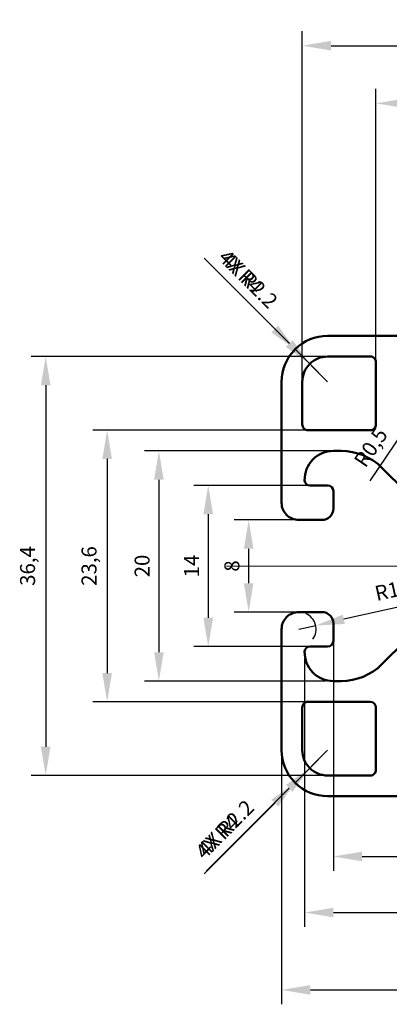
# Model space of a CAD drawing. Units: millimetres. Extents: x 2580.1 to 2672.5, y 2225.2 to 2310.7.
# Tile 1 of 2: x 2580.1 to 2612.2, y 2225.2 to 2310.7. Entities that reach past the tile are written whole.
import ezdxf

# ---------------------------------------------------------------- set-up
doc = ezdxf.new("R2010")
doc.units = ezdxf.units.MM
doc.linetypes.add('CENTER', pattern=[50.8, 31.75, -6.35, 6.35, -6.35])
for name, color, linetype, lineweight in [('M-CNTR', 1, 'CENTER', 18), ('M-DIMS', 2, 'Continuous', 25), ('M-OUTL', 7, 'Continuous', 50)]:
    doc.layers.add(name, color=color, linetype=linetype, lineweight=lineweight)
doc.styles.get("Standard").update_dxf_attribs({"font": 'arial.ttf'})
doc.dimstyles.new('ISO-25', dxfattribs={"dimtxt": 1.3, "dimasz": 2.5, "dimexe": 1.25, "dimexo": 0.625, "dimtad": 1, "dimtxsty": 'Standard', "dimcen": 2.5, "dimadec": 0, "dimazin": 0, "dimtfac": 1, "dimtmove": 0, "dimatfit": 3, "dimfxl": 1, "dimarcsym": 0})

# ---------------------------------------------------------------- blocks, each defined once
blk = doc.blocks.new('*D4')
at = {"layer": 'Defpoints', "color": 0, "transparency": 16777216}
for p in [(2634.649, 2303.442), (2611.049, 2278.243), (2634.649, 2278.243)]:
    blk.add_point(p, dxfattribs=at)
at = {"layer": 'M-DIMS', "color": 0, "lineweight": -2, "transparency": 16777216}
for p, q in [((2611.049, 2278.868), (2611.049, 2304.692)), ((2634.649, 2278.868), (2634.649, 2304.692)), ((2613.549, 2303.442), (2632.149, 2303.442))]:
    blk.add_line(p, q, dxfattribs=at)
at = {"layer": 'M-DIMS', "color": 0, "transparency": 16777216}
for points in [[(2613.549, 2303.859), (2613.549, 2303.026), (2611.049, 2303.442)], [(2632.149, 2303.859), (2632.149, 2303.026), (2634.649, 2303.442)]]:
    blk.add_solid(points, dxfattribs=at)
at = {"layer": 'M-DIMS', "color": 0, "transparency": 16777216, "insert": (2622.849, 2304.849), "char_height": 1.3, "attachment_point": 5}
blk.add_mtext('23,6', dxfattribs=at)
blk = doc.blocks.new('*D5')
at = {"layer": 'Defpoints', "color": 0, "transparency": 16777216}
for p in [(2641.049, 2308.452), (2604.649, 2277.393), (2641.049, 2277.393)]:
    blk.add_point(p, dxfattribs=at)
at = {"layer": 'M-DIMS', "color": 0, "lineweight": -2, "transparency": 16777216}
for p, q in [((2604.649, 2278.018), (2604.649, 2309.702)), ((2641.049, 2278.018), (2641.049, 2309.702)), ((2607.149, 2308.452), (2638.549, 2308.452))]:
    blk.add_line(p, q, dxfattribs=at)
at = {"layer": 'M-DIMS', "color": 0, "transparency": 16777216}
for points in [[(2607.149, 2308.869), (2607.149, 2308.036), (2604.649, 2308.452)], [(2638.549, 2308.869), (2638.549, 2308.036), (2641.049, 2308.452)]]:
    blk.add_solid(points, dxfattribs=at)
at = {"layer": 'M-DIMS', "color": 0, "transparency": 16777216, "insert": (2622.849, 2309.859), "char_height": 1.3, "attachment_point": 5}
blk.add_mtext('36,4', dxfattribs=at)
blk = doc.blocks.new('*D6')
at = {"layer": 'Defpoints', "color": 0, "transparency": 16777216}
for p in [(2608.699, 2281.443), (2582.357, 2245.043), (2608.699, 2245.043)]:
    blk.add_point(p, dxfattribs=at)
at = {"layer": 'M-DIMS', "color": 0, "lineweight": -2, "transparency": 16777216}
for p, q in [((2608.074, 2281.443), (2581.107, 2281.443)), ((2582.357, 2278.943), (2582.357, 2247.543)), ((2608.074, 2245.043), (2581.107, 2245.043))]:
    blk.add_line(p, q, dxfattribs=at)
at = {"layer": 'M-DIMS', "color": 0, "transparency": 16777216}
for points in [[(2581.941, 2278.943), (2582.774, 2278.943), (2582.357, 2281.443)], [(2581.941, 2247.543), (2582.774, 2247.543), (2582.357, 2245.043)]]:
    blk.add_solid(points, dxfattribs=at)
at = {"layer": 'M-DIMS', "color": 0, "transparency": 16777216, "insert": (2580.951, 2263.243), "char_height": 1.3, "attachment_point": 5, "rotation": 90}
blk.add_mtext('36,4', dxfattribs=at)
blk = doc.blocks.new('*D7')
at = {"layer": 'Defpoints', "color": 0, "transparency": 16777216}
for p in [(2605.349, 2267.243), (2599.989, 2259.243), (2605.349, 2259.243)]:
    blk.add_point(p, dxfattribs=at)
at = {"layer": 'M-DIMS', "color": 0, "lineweight": -2, "transparency": 16777216}
for p, q in [((2604.724, 2267.243), (2598.739, 2267.243)), ((2599.989, 2264.743), (2599.989, 2261.743)), ((2604.724, 2259.243), (2598.739, 2259.243))]:
    blk.add_line(p, q, dxfattribs=at)
at = {"layer": 'M-DIMS', "color": 0, "transparency": 16777216}
for points in [[(2599.572, 2264.743), (2600.405, 2264.743), (2599.989, 2267.243)], [(2599.572, 2261.743), (2600.405, 2261.743), (2599.989, 2259.243)]]:
    blk.add_solid(points, dxfattribs=at)
at = {"layer": 'M-DIMS', "color": 0, "transparency": 16777216, "insert": (2598.7, 2263.243), "char_height": 1.3, "attachment_point": 5, "rotation": 90}
blk.add_mtext('8', dxfattribs=at)
blk = doc.blocks.new('*D8')
at = {"layer": 'Defpoints', "color": 0, "transparency": 16777216}
for p in [(2606.075, 2270.243), (2596.476, 2256.243), (2606.075, 2256.243)]:
    blk.add_point(p, dxfattribs=at)
at = {"layer": 'M-DIMS', "color": 0, "lineweight": -2, "transparency": 16777216}
for p, q in [((2605.45, 2270.243), (2595.226, 2270.243)), ((2596.476, 2267.743), (2596.476, 2258.743)), ((2605.45, 2256.243), (2595.226, 2256.243))]:
    blk.add_line(p, q, dxfattribs=at)
at = {"layer": 'M-DIMS', "color": 0, "transparency": 16777216}
for points in [[(2596.06, 2267.743), (2596.893, 2267.743), (2596.476, 2270.243)], [(2596.06, 2258.743), (2596.893, 2258.743), (2596.476, 2256.243)]]:
    blk.add_solid(points, dxfattribs=at)
at = {"layer": 'M-DIMS', "color": 0, "transparency": 16777216, "insert": (2595.199, 2263.243), "char_height": 1.3, "attachment_point": 5, "rotation": 90}
blk.add_mtext('14', dxfattribs=at)
blk = doc.blocks.new('*D9')
at = {"layer": 'Defpoints', "color": 0, "transparency": 16777216}
for p in [(2607.689, 2273.243), (2592.189, 2253.244), (2607.301, 2253.244)]:
    blk.add_point(p, dxfattribs=at)
at = {"layer": 'M-DIMS', "color": 0, "lineweight": -2, "transparency": 16777216}
for p, q in [((2607.064, 2273.243), (2590.939, 2273.243)), ((2592.189, 2270.743), (2592.189, 2255.744)), ((2606.676, 2253.244), (2590.939, 2253.244))]:
    blk.add_line(p, q, dxfattribs=at)
at = {"layer": 'M-DIMS', "color": 0, "transparency": 16777216}
for points in [[(2591.773, 2270.743), (2592.606, 2270.743), (2592.189, 2273.243)], [(2591.773, 2255.744), (2592.606, 2255.744), (2592.189, 2253.244)]]:
    blk.add_solid(points, dxfattribs=at)
at = {"layer": 'M-DIMS', "color": 0, "transparency": 16777216, "insert": (2590.901, 2263.244), "char_height": 1.3, "attachment_point": 5, "rotation": 90}
blk.add_mtext('20', dxfattribs=at)
blk = doc.blocks.new('*D10')
at = {"layer": 'Defpoints', "color": 0, "transparency": 16777216}
for p in [(2607.849, 2275.043), (2587.696, 2251.443), (2607.849, 2251.443)]:
    blk.add_point(p, dxfattribs=at)
at = {"layer": 'M-DIMS', "color": 0, "lineweight": -2, "transparency": 16777216}
for p, q in [((2607.224, 2275.043), (2586.446, 2275.043)), ((2587.696, 2272.543), (2587.696, 2253.943)), ((2607.224, 2251.443), (2586.446, 2251.443))]:
    blk.add_line(p, q, dxfattribs=at)
at = {"layer": 'M-DIMS', "color": 0, "transparency": 16777216}
for points in [[(2587.279, 2272.543), (2588.113, 2272.543), (2587.696, 2275.043)], [(2587.279, 2253.943), (2588.113, 2253.943), (2587.696, 2251.443)]]:
    blk.add_solid(points, dxfattribs=at)
at = {"layer": 'M-DIMS', "color": 0, "transparency": 16777216, "insert": (2586.29, 2263.243), "char_height": 1.3, "attachment_point": 5, "rotation": 90}
blk.add_mtext('23,6', dxfattribs=at)
blk = doc.blocks.new('*D11')
at = {"layer": 'Defpoints', "color": 0, "transparency": 16777216}
for p in [(2602.849, 2247.243), (2642.849, 2247.243), (2642.849, 2226.409)]:
    blk.add_point(p, dxfattribs=at)
at = {"layer": 'M-DIMS', "color": 0, "lineweight": -2, "transparency": 16777216}
for p, q in [((2602.849, 2246.618), (2602.849, 2225.159)), ((2642.849, 2246.618), (2642.849, 2225.159)), ((2605.349, 2226.409), (2640.349, 2226.409))]:
    blk.add_line(p, q, dxfattribs=at)
at = {"layer": 'M-DIMS', "color": 0, "transparency": 16777216}
for points in [[(2605.349, 2226.826), (2605.349, 2225.992), (2602.849, 2226.409)], [(2640.349, 2226.826), (2640.349, 2225.992), (2642.849, 2226.409)]]:
    blk.add_solid(points, dxfattribs=at)
at = {"layer": 'M-DIMS', "color": 0, "transparency": 16777216, "insert": (2622.849, 2227.698), "char_height": 1.3, "attachment_point": 5}
blk.add_mtext('40', dxfattribs=at)
blk = doc.blocks.new('*D12')
at = {"layer": 'Defpoints', "color": 0, "transparency": 16777216}
for p in [(2607.349, 2257.493), (2638.349, 2257.493), (2638.349, 2238.001)]:
    blk.add_point(p, dxfattribs=at)
at = {"layer": 'M-DIMS', "color": 0, "lineweight": -2, "transparency": 16777216}
for p, q in [((2607.349, 2256.868), (2607.349, 2236.751)), ((2638.349, 2256.868), (2638.349, 2236.751)), ((2609.849, 2238.001), (2635.849, 2238.001))]:
    blk.add_line(p, q, dxfattribs=at)
at = {"layer": 'M-DIMS', "color": 0, "transparency": 16777216}
for points in [[(2609.849, 2238.418), (2609.849, 2237.584), (2607.349, 2238.001)], [(2635.849, 2238.418), (2635.849, 2237.584), (2638.349, 2238.001)]]:
    blk.add_solid(points, dxfattribs=at)
at = {"layer": 'M-DIMS', "color": 0, "transparency": 16777216, "insert": (2622.849, 2239.29), "char_height": 1.3, "attachment_point": 5}
blk.add_mtext('31', dxfattribs=at)
blk = doc.blocks.new('*D13')
at = {"layer": 'Defpoints', "color": 0, "transparency": 16777216}
for p in [(2604.85, 2255.804), (2640.849, 2255.743), (2640.849, 2233.131)]:
    blk.add_point(p, dxfattribs=at)
at = {"layer": 'M-DIMS', "color": 0, "lineweight": -2, "transparency": 16777216}
for p, q in [((2604.85, 2255.179), (2604.85, 2231.881)), ((2640.849, 2255.118), (2640.849, 2231.881)), ((2607.35, 2233.131), (2638.349, 2233.131))]:
    blk.add_line(p, q, dxfattribs=at)
at = {"layer": 'M-DIMS', "color": 0, "transparency": 16777216}
for points in [[(2607.35, 2233.547), (2607.35, 2232.714), (2604.85, 2233.131)], [(2638.349, 2233.547), (2638.349, 2232.714), (2640.849, 2233.131)]]:
    blk.add_solid(points, dxfattribs=at)
at = {"layer": 'M-DIMS', "color": 0, "transparency": 16777216, "insert": (2622.85, 2234.42), "char_height": 1.3, "attachment_point": 5}
blk.add_mtext('36', dxfattribs=at)
blk = doc.blocks.new('*D18')
at = {"layer": 'Defpoints', "color": 0, "transparency": 16777216}
for p in [(2616.349, 2279.243), (2616.069, 2278.829)]:
    blk.add_point(p, dxfattribs=at)
at = {"layer": 'M-DIMS', "color": 0, "lineweight": -2, "transparency": 16777216}
for p, q in [((2616.349, 2279.243), (2616.069, 2278.829)), ((2610.54, 2270.653), (2614.669, 2276.758))]:
    blk.add_line(p, q, dxfattribs=at)
at = {"layer": 'M-DIMS', "color": 0, "transparency": 16777216}
blk.add_solid([(2614.324, 2276.992), (2615.014, 2276.525), (2616.069, 2278.829)], dxfattribs=at)
at = {"layer": 'M-DIMS', "color": 0, "transparency": 16777216, "insert": (2610.739, 2273.458), "char_height": 1.3, "attachment_point": 5, "rotation": 55.93249}
blk.add_mtext('R0,5', dxfattribs=at)
blk = doc.blocks.new('*D24')
at = {"layer": 'Defpoints', "color": 0, "transparency": 16777216}
for p in [(2604.349, 2257.743), (2605.814, 2258.069)]:
    blk.add_point(p, dxfattribs=at)
at = {"layer": 'M-DIMS', "color": 0, "lineweight": -2, "transparency": 16777216}
for p, q in [((2615.449, 2260.209), (2608.254, 2258.611)), ((2604.349, 2257.743), (2605.814, 2258.069))]:
    blk.add_line(p, q, dxfattribs=at)
blk.add_arc((2604.349, 2257.743), 1.5, 324.77892, 66.12676, dxfattribs=at)
at = {"layer": 'M-DIMS', "color": 0, "transparency": 16777216}
blk.add_solid([(2608.164, 2259.018), (2608.345, 2258.204), (2605.814, 2258.069)], dxfattribs=at)
at = {"layer": 'M-DIMS', "color": 0, "transparency": 16777216, "insert": (2612.767, 2261.054), "char_height": 1.3, "attachment_point": 5, "rotation": 12.5254}
blk.add_mtext('R1,5', dxfattribs=at)
blk = doc.blocks.new('*D35')
at = {"layer": 'Defpoints', "color": 0, "transparency": 16777216}
for p in [(2606.849, 2247.243), (2604.023, 2244.413)]:
    blk.add_point(p, dxfattribs=at)
at = {"layer": 'M-DIMS', "color": 0, "lineweight": -2, "transparency": 16777216}
for p, q in [((2606.849, 2247.243), (2604.023, 2244.413)), ((2596.118, 2236.497), (2602.256, 2242.644))]:
    blk.add_line(p, q, dxfattribs=at)
at = {"layer": 'M-DIMS', "color": 0, "transparency": 16777216}
blk.add_solid([(2601.962, 2242.938), (2602.551, 2242.35), (2604.023, 2244.413)], dxfattribs=at)
at = {"layer": 'M-DIMS', "color": 0, "transparency": 16777216, "insert": (2597.402, 2239.587), "char_height": 1.3, "attachment_point": 5, "rotation": 45.04}
blk.add_mtext('4X R4', dxfattribs=at)
blk = doc.blocks.new('*D36')
at = {"layer": 'Defpoints', "color": 0, "transparency": 16777216}
for p in [(2606.849, 2247.243), (2605.291, 2245.691)]:
    blk.add_point(p, dxfattribs=at)
at = {"layer": 'M-DIMS', "color": 0, "lineweight": -2, "transparency": 16777216}
for p, q in [((2606.849, 2247.243), (2605.291, 2245.691)), ((2596.298, 2236.733), (2603.52, 2243.926))]:
    blk.add_line(p, q, dxfattribs=at)
at = {"layer": 'M-DIMS', "color": 0, "transparency": 16777216}
blk.add_solid([(2603.226, 2244.222), (2603.814, 2243.631), (2605.291, 2245.691)], dxfattribs=at)
at = {"layer": 'M-DIMS', "color": 0, "transparency": 16777216, "insert": (2598.121, 2240.353), "char_height": 1.3, "attachment_point": 5, "rotation": 44.88871}
blk.add_mtext('4X R2.2', dxfattribs=at)
blk = doc.blocks.new('*D37')
at = {"layer": 'Defpoints', "color": 0, "transparency": 16777216}
for p in [(2604.021, 2282.072), (2606.849, 2279.243)]:
    blk.add_point(p, dxfattribs=at)
at = {"layer": 'M-DIMS', "color": 0, "lineweight": -2, "transparency": 16777216}
for p, q in [((2596.111, 2289.982), (2602.253, 2283.84)), ((2606.849, 2279.243), (2604.021, 2282.072))]:
    blk.add_line(p, q, dxfattribs=at)
at = {"layer": 'M-DIMS', "color": 0, "transparency": 16777216}
blk.add_solid([(2602.548, 2284.134), (2601.959, 2283.545), (2604.021, 2282.072)], dxfattribs=at)
at = {"layer": 'M-DIMS', "color": 0, "transparency": 16777216, "insert": (2599.2, 2288.697), "char_height": 1.3, "attachment_point": 5, "rotation": 314.99783}
blk.add_mtext('4X R4', dxfattribs=at)
blk = doc.blocks.new('*D38')
at = {"layer": 'Defpoints', "color": 0, "transparency": 16777216}
for p in [(2605.294, 2280.799), (2606.849, 2279.243)]:
    blk.add_point(p, dxfattribs=at)
at = {"layer": 'M-DIMS', "color": 0, "lineweight": -2, "transparency": 16777216}
for p, q in [((2596.319, 2289.775), (2603.526, 2282.567)), ((2606.849, 2279.243), (2605.294, 2280.799))]:
    blk.add_line(p, q, dxfattribs=at)
at = {"layer": 'M-DIMS', "color": 0, "transparency": 16777216}
blk.add_solid([(2603.821, 2282.862), (2603.232, 2282.272), (2605.294, 2280.799)], dxfattribs=at)
at = {"layer": 'M-DIMS', "color": 0, "transparency": 16777216, "insert": (2599.943, 2287.959), "char_height": 1.3, "attachment_point": 5, "rotation": 314.99606}
blk.add_mtext('4X R2.2', dxfattribs=at)

msp = doc.modelspace()

# ---------------------------------------------------------------- linework, layer by layer
at = {"layer": 'M-CNTR'}
msp.add_line((2598.059, 2263.243), (2646.996, 2263.243), dxfattribs=at)
at = {"layer": 'M-OUTL'}
for p, q in [((2607.349, 2273.243), (2608.028, 2273.243)), ((2613.635, 2269.708), (2611.564, 2271.779)), ((2606.849, 2270.243), (2605.3, 2270.243)), ((2607.349, 2258.243), (2607.349, 2256.743)), ((2606.849, 2256.243), (2605.3, 2256.243)), ((2613.635, 2256.779), (2611.564, 2254.708)), ((2607.349, 2253.243), (2608.028, 2253.243))]:
    msp.add_line(p, q, dxfattribs=at)
for points in [[(2607.349, 2269.743), (2607.349, 2268.243, -0.414214), (2606.349, 2267.243), (2604.349, 2267.243, -0.414214), (2602.849, 2268.743), (2602.849, 2279.243, -0.414214), (2606.849, 2283.243), (2617.349, 2283.243)], [(2618.849, 2246.743), (2618.849, 2244.743, -0.414214), (2617.349, 2243.243), (2606.849, 2243.243, -0.414214), (2602.849, 2247.243), (2602.849, 2257.743, -0.414214), (2604.349, 2259.243), (2606.349, 2259.243)], [(2611.049, 2250.943), (2611.049, 2245.543, -0.414214), (2610.549, 2245.043), (2606.849, 2245.043, -0.414214), (2604.649, 2247.243), (2604.649, 2250.943, -0.414214), (2605.149, 2251.443), (2610.549, 2251.443)]]:
    msp.add_lwpolyline(points, format="xyb", dxfattribs=at)
msp.add_lwpolyline([(2610.549, 2275.043), (2605.149, 2275.043, -0.414214), (2604.649, 2275.543), (2604.649, 2279.243, -0.414214), (2606.849, 2281.443), (2610.549, 2281.443, -0.414214), (2611.049, 2280.943), (2611.049, 2275.543, -0.414214)], format="xyb", close=True, dxfattribs=at)
for centre, radius, start, end in [((2607.349, 2270.743), 2.5, 90, 181.3976), ((2608.028, 2268.243), 5, 45, 90), ((2605.3, 2270.693), 0.45, 181.3976, 270), ((2606.849, 2269.743), 0.5, 0, 90), ((2606.349, 2258.243), 1, 0, 90), ((2605.3, 2255.793), 0.45, 90, 178.6024), ((2606.849, 2256.743), 0.5, 270, 0), ((2607.349, 2255.743), 2.5, 178.6024, 270), ((2608.028, 2258.243), 5, 270, 315), ((2610.549, 2250.943), 0.5, 0, 90)]:
    msp.add_arc(centre, radius, start, end, dxfattribs=at)

# ---------------------------------------------------------------- dimensions: what is measured, and where the dimension line sits
at = {"layer": 'M-DIMS'}
for base, p1, p2, picture, middle in [((2641.049, 2308.452), (2604.649, 2277.393), (2641.049, 2277.393), '*D5', (2622.849, 2309.859)), ((2634.649, 2303.442), (2611.049, 2278.243), (2634.649, 2278.243), '*D4', (2622.849, 2304.849)), ((2638.349, 2238.001), (2607.349, 2257.493), (2638.349, 2257.493), '*D12', (2622.849, 2239.29)), ((2640.849, 2233.131), (2604.85, 2255.804), (2640.849, 2255.743), '*D13', (2622.85, 2234.42)), ((2642.849, 2226.409), (2602.849, 2247.243), (2642.849, 2247.243), '*D11', (2622.849, 2227.698))]:
    dim = msp.add_linear_dim(base=base, p1=p1, p2=p2, dimstyle='ISO-25', override={"dimclrd": 0, "dimclre": 0, "dimclrt": 0}, dxfattribs=at)
    dim.commit()
    dim.dimension.update_dxf_attribs({"geometry": picture, "text_midpoint": middle})
for center, mpoint, override, picture, middle in [((2606.849, 2279.243), (2604.021, 2282.072), {"dimdec": 0, "dimlfac": 1, "dimrnd": 0, "dimzin": 0, "dimdsep": 46, "dimlunit": 2}, '*D37', (2599.2, 2288.697)), ((2606.849, 2279.243), (2605.294, 2280.799), {"dimdec": 1, "dimlfac": 1, "dimrnd": 0, "dimzin": 0, "dimdsep": 46, "dimlunit": 2}, '*D38', (2599.943, 2287.959)), ((2606.849, 2247.243), (2604.023, 2244.413), {"dimdec": 0, "dimlfac": 1, "dimrnd": 0, "dimzin": 0, "dimdsep": 46, "dimlunit": 2}, '*D35', (2597.402, 2239.587)), ((2606.849, 2247.243), (2605.291, 2245.691), {"dimdec": 1, "dimlfac": 1, "dimrnd": 0, "dimzin": 0, "dimdsep": 46, "dimlunit": 2}, '*D36', (2598.121, 2240.353))]:
    dim = msp.add_radius_dim(center=center, mpoint=mpoint, text='4X <>', dimstyle='ISO-25', override=override, dxfattribs=at)
    dim.commit()
    dim.dimension.update_dxf_attribs({"geometry": picture, "text_midpoint": middle})
for base, p1, p2, picture, middle in [((2582.357, 2245.043), (2608.699, 2281.443), (2608.699, 2245.043), '*D6', (2580.951, 2263.243)), ((2587.696, 2251.443), (2607.849, 2275.043), (2607.849, 2251.443), '*D10', (2586.29, 2263.243)), ((2592.189, 2253.244), (2607.689, 2273.243), (2607.301, 2253.244), '*D9', (2590.901, 2263.244)), ((2596.476, 2256.243), (2606.075, 2270.243), (2606.075, 2256.243), '*D8', (2595.199, 2263.243)), ((2599.989, 2259.243), (2605.349, 2267.243), (2605.349, 2259.243), '*D7', (2598.7, 2263.243))]:
    dim = msp.add_linear_dim(base=base, p1=p1, p2=p2, angle=90, dimstyle='ISO-25', override={"dimclrd": 0, "dimclre": 0, "dimclrt": 0}, dxfattribs=at)
    dim.commit()
    dim.dimension.update_dxf_attribs({"geometry": picture, "text_midpoint": middle})
for center, mpoint, picture, middle in [((2616.349, 2279.243), (2616.069, 2278.829), '*D18', (2610.739, 2273.458)), ((2604.349, 2257.743), (2605.814, 2258.069), '*D24', (2612.767, 2261.054))]:
    dim = msp.add_radius_dim(center=center, mpoint=mpoint, dimstyle='ISO-25', override={"dimclrd": 0, "dimclre": 0, "dimclrt": 0}, dxfattribs=at)
    dim.commit()
    dim.dimension.update_dxf_attribs({"geometry": picture, "text_midpoint": middle})

doc.saveas('drawing.dxf')
